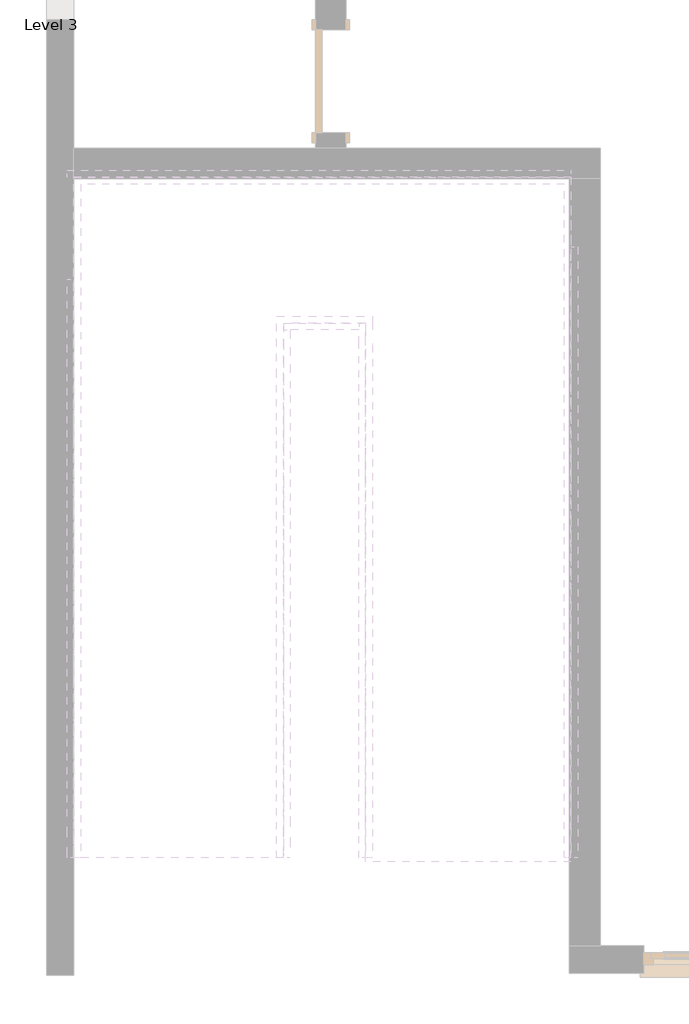
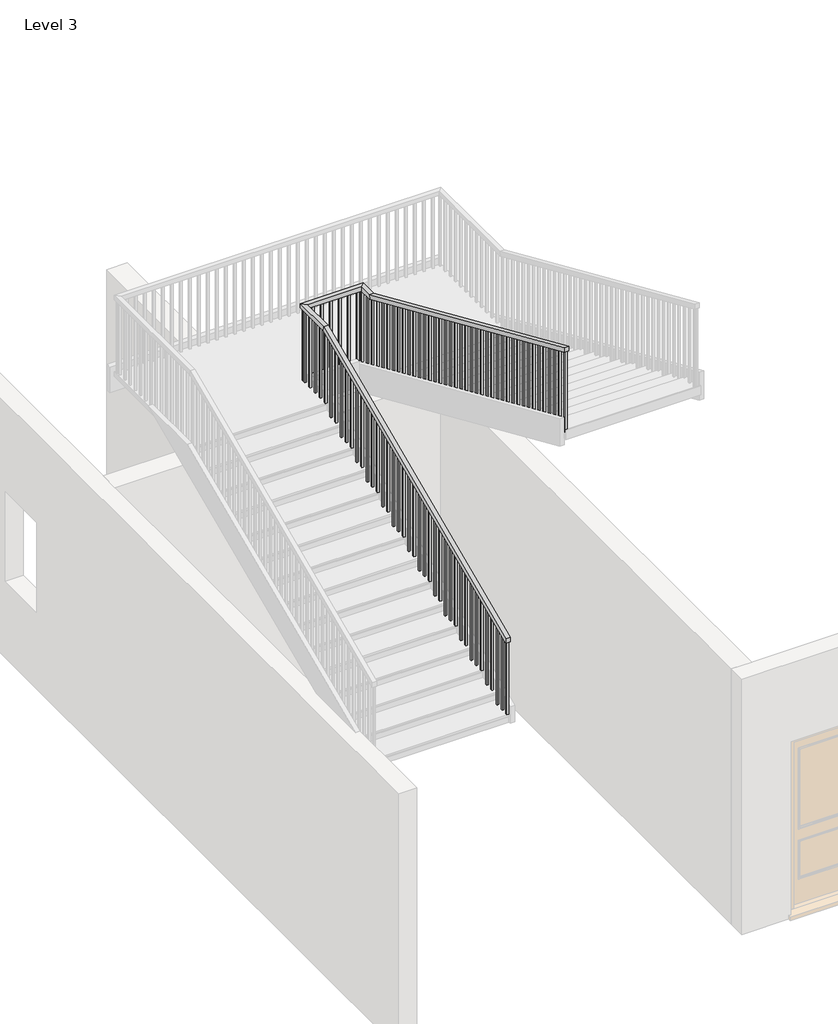
# One storey, part 2 of 6: 1 railing.
"""IFC4 building model written with IfcOpenShell, lengths in millimetres."""

from ifc_helpers import new_model, si_unit, frame, origin, place, context, project, spatial, polyline, outline, extrude, faceted_brep, element, save

model = new_model("IFC4")

# Units and contexts
model_context = context("Model", 3, world=origin())
ifc_project = project(units=[si_unit("LENGTHUNIT", "METRE", prefix="MILLI")], contexts=[model_context])

# Site, building, storey
site = spatial("IfcSite", under=ifc_project)
building = spatial("IfcBuilding", under=site)
storey = spatial("IfcBuildingStorey", under=building, Name="Level 3", Elevation=6096.0)

# Railing
placement = place(None, origin())
element("IfcRailing", 1, ObjectType="Handrail - Rectangular", at=placement, inside=storey, context=model_context, shape_type="SolidModel", body=[
    faceted_brep([(-6050.7290366, -6973.0610642, 9865.36), (-6050.7290366, -6973.0610642, 9809.8599828), (-5999.9290366, -6973.0610642, 9809.8599828), (-5999.9290366, -6973.0610642, 9865.36), (-6050.7290366, -3417.0610642, 11430.0), (-6050.7290366, -3406.3792071, 11379.2), (-5999.9290366, -3406.3792071, 11379.2), (-5999.9290366, -3417.0610642, 11430.0), (-6050.7290366, -2959.8610642, 11430.0), (-6050.7290366, -2959.8610642, 11379.2), (-5999.9290366, -3010.6610642, 11379.2), (-5999.9290366, -3010.6610642, 11430.0), (-5339.5290366, -2959.8610642, 11430.0), (-5339.5290366, -2959.8610642, 11379.2), (-5390.3290366, -3010.6610642, 11379.2), (-5390.3290366, -3010.6610642, 11430.0), (-5339.5290366, -3163.0610642, 11430.0), (-5339.5290366, -3173.7429214, 11379.2), (-5390.3290366, -3173.7429214, 11379.2), (-5390.3290366, -3163.0610642, 11430.0), (-5339.5290366, -6973.0610642, 13106.4), (-5390.3290366, -6973.0610642, 13106.4), (-5390.3290366, -6973.0610642, 13050.8999828), (-5339.5290366, -6973.0610642, 13050.8999828)], [[[0, 1, 2, 3]], [[1, 0, 4, 5]], [[2, 1, 5, 6]], [[3, 2, 6, 7]], [[0, 3, 7, 4]], [[5, 4, 8, 9]], [[6, 5, 9, 10]], [[7, 6, 10, 11]], [[4, 7, 11, 8]], [[9, 8, 12, 13]], [[10, 9, 13, 14]], [[11, 10, 14, 15]], [[8, 11, 15, 12]], [[13, 12, 16, 17]], [[14, 13, 17, 18]], [[15, 14, 18, 19]], [[12, 15, 19, 16]], [[20, 21, 22, 23]], [[17, 16, 20, 23]], [[18, 17, 23, 22]], [[19, 18, 22, 21]], [[16, 19, 21, 20]]]),
    extrude(outline(polyline([(-6957.1860642, 13043.9149828), (-6938.1360642, 13035.5329828), (-6938.1360642, 12080.24), (-6957.1860642, 12080.24), (-6957.1860642, 13043.9149828)])), frame((-5374.4540366, 0.0, 0.0), z_axis=(1.0, 0.0, 0.0), x_axis=(0.0, 1.0, 0.0)), (0.0, 0.0, 1.0), 19.05),
    extrude(outline(polyline([(-6855.5860642, 12999.2109828), (-6836.5360642, 12990.8289828), (-6836.5360642, 12080.24), (-6855.5860642, 12080.24), (-6855.5860642, 12999.2109828)])), frame((-5374.4540366, 0.0, 0.0), z_axis=(1.0, 0.0, 0.0), x_axis=(0.0, 1.0, 0.0)), (0.0, 0.0, 1.0), 19.05),
    extrude(outline(polyline([(-6753.9860642, 12954.5069828), (-6734.9360642, 12946.1249828), (-6734.9360642, 12080.24), (-6753.9860642, 12080.24), (-6753.9860642, 12954.5069828)])), frame((-5374.4540366, 0.0, 0.0), z_axis=(1.0, 0.0, 0.0), x_axis=(0.0, 1.0, 0.0)), (0.0, 0.0, 1.0), 19.05),
    extrude(outline(polyline([(-6652.3860642, 12909.8029828), (-6633.3360642, 12901.4209828), (-6633.3360642, 11968.48), (-6652.3860642, 11968.48), (-6652.3860642, 12909.8029828)])), frame((-5374.4540366, 0.0, 0.0), z_axis=(1.0, 0.0, 0.0), x_axis=(0.0, 1.0, 0.0)), (0.0, 0.0, 1.0), 19.05),
    extrude(outline(polyline([(-6550.7860642, 12865.0989828), (-6531.7360642, 12856.7169828), (-6531.7360642, 11968.48), (-6550.7860642, 11968.48), (-6550.7860642, 12865.0989828)])), frame((-5374.4540366, 0.0, 0.0), z_axis=(1.0, 0.0, 0.0), x_axis=(0.0, 1.0, 0.0)), (0.0, 0.0, 1.0), 19.05),
    extrude(outline(polyline([(-6449.1860642, 12820.3949828), (-6430.1360642, 12812.0129828), (-6430.1360642, 11856.72), (-6449.1860642, 11856.72), (-6449.1860642, 12820.3949828)])), frame((-5374.4540366, 0.0, 0.0), z_axis=(1.0, 0.0, 0.0), x_axis=(0.0, 1.0, 0.0)), (0.0, 0.0, 1.0), 19.05),
    extrude(outline(polyline([(-6347.5860642, 12775.6909828), (-6328.5360642, 12767.3089828), (-6328.5360642, 11856.72), (-6347.5860642, 11856.72), (-6347.5860642, 12775.6909828)])), frame((-5374.4540366, 0.0, 0.0), z_axis=(1.0, 0.0, 0.0), x_axis=(0.0, 1.0, 0.0)), (0.0, 0.0, 1.0), 19.05),
    extrude(outline(polyline([(-6245.9860642, 12730.9869828), (-6226.9360642, 12722.6049828), (-6226.9360642, 11856.72), (-6245.9860642, 11856.72), (-6245.9860642, 12730.9869828)])), frame((-5374.4540366, 0.0, 0.0), z_axis=(1.0, 0.0, 0.0), x_axis=(0.0, 1.0, 0.0)), (0.0, 0.0, 1.0), 19.05),
    extrude(outline(polyline([(-6144.3860642, 12686.2829828), (-6125.3360642, 12677.9009828), (-6125.3360642, 11744.96), (-6144.3860642, 11744.96), (-6144.3860642, 12686.2829828)])), frame((-5374.4540366, 0.0, 0.0), z_axis=(1.0, 0.0, 0.0), x_axis=(0.0, 1.0, 0.0)), (0.0, 0.0, 1.0), 19.05),
    extrude(outline(polyline([(-6042.7860642, 12641.5789828), (-6023.7360642, 12633.1969828), (-6023.7360642, 11744.96), (-6042.7860642, 11744.96), (-6042.7860642, 12641.5789828)])), frame((-5374.4540366, 0.0, 0.0), z_axis=(1.0, 0.0, 0.0), x_axis=(0.0, 1.0, 0.0)), (0.0, 0.0, 1.0), 19.05),
    extrude(outline(polyline([(-5941.1860642, 12596.8749828), (-5922.1360642, 12588.4929828), (-5922.1360642, 11633.2), (-5941.1860642, 11633.2), (-5941.1860642, 12596.8749828)])), frame((-5374.4540366, 0.0, 0.0), z_axis=(1.0, 0.0, 0.0), x_axis=(0.0, 1.0, 0.0)), (0.0, 0.0, 1.0), 19.05),
    extrude(outline(polyline([(-5839.5860642, 12552.1709828), (-5820.5360642, 12543.7889828), (-5820.5360642, 11633.2), (-5839.5860642, 11633.2), (-5839.5860642, 12552.1709828)])), frame((-5374.4540366, 0.0, 0.0), z_axis=(1.0, 0.0, 0.0), x_axis=(0.0, 1.0, 0.0)), (0.0, 0.0, 1.0), 19.05),
    extrude(outline(polyline([(-5737.9860642, 12507.4669828), (-5718.9360642, 12499.0849828), (-5718.9360642, 11633.2), (-5737.9860642, 11633.2), (-5737.9860642, 12507.4669828)])), frame((-5374.4540366, 0.0, 0.0), z_axis=(1.0, 0.0, 0.0), x_axis=(0.0, 1.0, 0.0)), (0.0, 0.0, 1.0), 19.05),
    extrude(outline(polyline([(-5636.3860642, 12462.7629828), (-5617.3360642, 12454.3809828), (-5617.3360642, 11521.44), (-5636.3860642, 11521.44), (-5636.3860642, 12462.7629828)])), frame((-5374.4540366, 0.0, 0.0), z_axis=(1.0, 0.0, 0.0), x_axis=(0.0, 1.0, 0.0)), (0.0, 0.0, 1.0), 19.05),
    extrude(outline(polyline([(-5534.7860642, 12418.0589828), (-5515.7360642, 12409.6769828), (-5515.7360642, 11521.44), (-5534.7860642, 11521.44), (-5534.7860642, 12418.0589828)])), frame((-5374.4540366, 0.0, 0.0), z_axis=(1.0, 0.0, 0.0), x_axis=(0.0, 1.0, 0.0)), (0.0, 0.0, 1.0), 19.05),
    extrude(outline(polyline([(-5433.1860642, 12373.3549828), (-5414.1360642, 12364.9729828), (-5414.1360642, 11409.68), (-5433.1860642, 11409.68), (-5433.1860642, 12373.3549828)])), frame((-5374.4540366, 0.0, 0.0), z_axis=(1.0, 0.0, 0.0), x_axis=(0.0, 1.0, 0.0)), (0.0, 0.0, 1.0), 19.05),
    extrude(outline(polyline([(-5331.5860642, 12328.6509828), (-5312.5360642, 12320.2689828), (-5312.5360642, 11409.68), (-5331.5860642, 11409.68), (-5331.5860642, 12328.6509828)])), frame((-5374.4540366, 0.0, 0.0), z_axis=(1.0, 0.0, 0.0), x_axis=(0.0, 1.0, 0.0)), (0.0, 0.0, 1.0), 19.05),
    extrude(outline(polyline([(-5229.9860642, 12283.9469828), (-5210.9360642, 12275.5649828), (-5210.9360642, 11409.68), (-5229.9860642, 11409.68), (-5229.9860642, 12283.9469828)])), frame((-5374.4540366, 0.0, 0.0), z_axis=(1.0, 0.0, 0.0), x_axis=(0.0, 1.0, 0.0)), (0.0, 0.0, 1.0), 19.05),
    extrude(outline(polyline([(-5128.3860642, 12239.2429828), (-5109.3360642, 12230.8609828), (-5109.3360642, 11297.92), (-5128.3860642, 11297.92), (-5128.3860642, 12239.2429828)])), frame((-5374.4540366, 0.0, 0.0), z_axis=(1.0, 0.0, 0.0), x_axis=(0.0, 1.0, 0.0)), (0.0, 0.0, 1.0), 19.05),
    extrude(outline(polyline([(-5026.7860642, 12194.5389828), (-5007.7360642, 12186.1569828), (-5007.7360642, 11297.92), (-5026.7860642, 11297.92), (-5026.7860642, 12194.5389828)])), frame((-5374.4540366, 0.0, 0.0), z_axis=(1.0, 0.0, 0.0), x_axis=(0.0, 1.0, 0.0)), (0.0, 0.0, 1.0), 19.05),
    extrude(outline(polyline([(-4925.1860642, 12149.8349828), (-4906.1360642, 12141.4529828), (-4906.1360642, 11186.16), (-4925.1860642, 11186.16), (-4925.1860642, 12149.8349828)])), frame((-5374.4540366, 0.0, 0.0), z_axis=(1.0, 0.0, 0.0), x_axis=(0.0, 1.0, 0.0)), (0.0, 0.0, 1.0), 19.05),
    extrude(outline(polyline([(-4823.5860642, 12105.1309828), (-4804.5360642, 12096.7489828), (-4804.5360642, 11186.16), (-4823.5860642, 11186.16), (-4823.5860642, 12105.1309828)])), frame((-5374.4540366, 0.0, 0.0), z_axis=(1.0, 0.0, 0.0), x_axis=(0.0, 1.0, 0.0)), (0.0, 0.0, 1.0), 19.05),
    extrude(outline(polyline([(-4721.9860642, 12060.4269828), (-4702.9360642, 12052.0449828), (-4702.9360642, 11186.16), (-4721.9860642, 11186.16), (-4721.9860642, 12060.4269828)])), frame((-5374.4540366, 0.0, 0.0), z_axis=(1.0, 0.0, 0.0), x_axis=(0.0, 1.0, 0.0)), (0.0, 0.0, 1.0), 19.05),
    extrude(outline(polyline([(-4620.3860642, 12015.7229828), (-4601.3360642, 12007.3409828), (-4601.3360642, 11074.4), (-4620.3860642, 11074.4), (-4620.3860642, 12015.7229828)])), frame((-5374.4540366, 0.0, 0.0), z_axis=(1.0, 0.0, 0.0), x_axis=(0.0, 1.0, 0.0)), (0.0, 0.0, 1.0), 19.05),
    extrude(outline(polyline([(-4518.7860642, 11971.0189828), (-4499.7360642, 11962.6369828), (-4499.7360642, 11074.4), (-4518.7860642, 11074.4), (-4518.7860642, 11971.0189828)])), frame((-5374.4540366, 0.0, 0.0), z_axis=(1.0, 0.0, 0.0), x_axis=(0.0, 1.0, 0.0)), (0.0, 0.0, 1.0), 19.05),
    extrude(outline(polyline([(-4417.1860642, 11926.3149828), (-4398.1360642, 11917.9329828), (-4398.1360642, 10962.64), (-4417.1860642, 10962.64), (-4417.1860642, 11926.3149828)])), frame((-5374.4540366, 0.0, 0.0), z_axis=(1.0, 0.0, 0.0), x_axis=(0.0, 1.0, 0.0)), (0.0, 0.0, 1.0), 19.05),
    extrude(outline(polyline([(-4315.5860642, 11881.6109828), (-4296.5360642, 11873.2289828), (-4296.5360642, 10962.64), (-4315.5860642, 10962.64), (-4315.5860642, 11881.6109828)])), frame((-5374.4540366, 0.0, 0.0), z_axis=(1.0, 0.0, 0.0), x_axis=(0.0, 1.0, 0.0)), (0.0, 0.0, 1.0), 19.05),
    extrude(outline(polyline([(-4213.9860642, 11836.9069828), (-4194.9360642, 11828.5249828), (-4194.9360642, 10962.64), (-4213.9860642, 10962.64), (-4213.9860642, 11836.9069828)])), frame((-5374.4540366, 0.0, 0.0), z_axis=(1.0, 0.0, 0.0), x_axis=(0.0, 1.0, 0.0)), (0.0, 0.0, 1.0), 19.05),
    extrude(outline(polyline([(-4112.3860642, 11792.2029828), (-4093.3360642, 11783.8209828), (-4093.3360642, 10850.88), (-4112.3860642, 10850.88), (-4112.3860642, 11792.2029828)])), frame((-5374.4540366, 0.0, 0.0), z_axis=(1.0, 0.0, 0.0), x_axis=(0.0, 1.0, 0.0)), (0.0, 0.0, 1.0), 19.05),
    extrude(outline(polyline([(-4010.7860642, 11747.4989828), (-3991.7360642, 11739.1169828), (-3991.7360642, 10850.88), (-4010.7860642, 10850.88), (-4010.7860642, 11747.4989828)])), frame((-5374.4540366, 0.0, 0.0), z_axis=(1.0, 0.0, 0.0), x_axis=(0.0, 1.0, 0.0)), (0.0, 0.0, 1.0), 19.05),
    extrude(outline(polyline([(-3909.1860642, 11702.7949828), (-3890.1360642, 11694.4129828), (-3890.1360642, 10739.12), (-3909.1860642, 10739.12), (-3909.1860642, 11702.7949828)])), frame((-5374.4540366, 0.0, 0.0), z_axis=(1.0, 0.0, 0.0), x_axis=(0.0, 1.0, 0.0)), (0.0, 0.0, 1.0), 19.05),
    extrude(outline(polyline([(-3807.5860642, 11658.0909828), (-3788.5360642, 11649.7089828), (-3788.5360642, 10739.12), (-3807.5860642, 10739.12), (-3807.5860642, 11658.0909828)])), frame((-5374.4540366, 0.0, 0.0), z_axis=(1.0, 0.0, 0.0), x_axis=(0.0, 1.0, 0.0)), (0.0, 0.0, 1.0), 19.05),
    extrude(outline(polyline([(-3705.9860642, 11613.3869828), (-3686.9360642, 11605.0049828), (-3686.9360642, 10739.12), (-3705.9860642, 10739.12), (-3705.9860642, 11613.3869828)])), frame((-5374.4540366, 0.0, 0.0), z_axis=(1.0, 0.0, 0.0), x_axis=(0.0, 1.0, 0.0)), (0.0, 0.0, 1.0), 19.05),
    extrude(outline(polyline([(-3604.3860642, 11568.6829828), (-3585.3360642, 11560.3009828), (-3585.3360642, 10627.36), (-3604.3860642, 10627.36), (-3604.3860642, 11568.6829828)])), frame((-5374.4540366, 0.0, 0.0), z_axis=(1.0, 0.0, 0.0), x_axis=(0.0, 1.0, 0.0)), (0.0, 0.0, 1.0), 19.05),
    extrude(outline(polyline([(-3502.7860642, 11523.9789828), (-3483.7360642, 11515.5969828), (-3483.7360642, 10627.36), (-3502.7860642, 10627.36), (-3502.7860642, 11523.9789828)])), frame((-5374.4540366, 0.0, 0.0), z_axis=(1.0, 0.0, 0.0), x_axis=(0.0, 1.0, 0.0)), (0.0, 0.0, 1.0), 19.05),
    extrude(outline(polyline([(-3401.1860642, 11479.2749828), (-3382.1360642, 11470.8929828), (-3382.1360642, 10515.6), (-3401.1860642, 10515.6), (-3401.1860642, 11479.2749828)])), frame((-5374.4540366, 0.0, 0.0), z_axis=(1.0, 0.0, 0.0), x_axis=(0.0, 1.0, 0.0)), (0.0, 0.0, 1.0), 19.05),
    extrude(outline(polyline([(-3299.5860642, 11434.5709828), (-3280.5360642, 11426.1889828), (-3280.5360642, 10515.6), (-3299.5860642, 10515.6), (-3299.5860642, 11434.5709828)])), frame((-5374.4540366, 0.0, 0.0), z_axis=(1.0, 0.0, 0.0), x_axis=(0.0, 1.0, 0.0)), (0.0, 0.0, 1.0), 19.05),
    extrude(outline(polyline([(-3197.9860642, 11389.8669828), (-3178.9360642, 11381.4849828), (-3178.9360642, 10515.6), (-3197.9860642, 10515.6), (-3197.9860642, 11389.8669828)])), frame((-5374.4540366, 0.0, 0.0), z_axis=(1.0, 0.0, 0.0), x_axis=(0.0, 1.0, 0.0)), (0.0, 0.0, 1.0), 19.05),
    extrude(outline(polyline([(-5374.4540366, -3077.3360642), (-5355.4040366, -3077.3360642), (-5355.4040366, -3096.3860642), (-5374.4540366, -3096.3860642), (-5374.4540366, -3077.3360642)])), frame((0.0, 0.0, 10515.6), z_axis=(0.0, 0.0, 1.0), x_axis=(1.0, 0.0, 0.0)), (0.0, 0.0, 1.0), 863.6),
    extrude(outline(polyline([(-5425.2540366, -2994.7860642), (-5425.2540366, -2975.7360642), (-5406.2040366, -2975.7360642), (-5406.2040366, -2994.7860642), (-5425.2540366, -2994.7860642)])), frame((0.0, 0.0, 10515.6), z_axis=(0.0, 0.0, 1.0), x_axis=(1.0, 0.0, 0.0)), (0.0, 0.0, 1.0), 863.6),
    extrude(outline(polyline([(-5526.8540366, -2994.7860642), (-5526.8540366, -2975.7360642), (-5507.8040366, -2975.7360642), (-5507.8040366, -2994.7860642), (-5526.8540366, -2994.7860642)])), frame((0.0, 0.0, 10515.6), z_axis=(0.0, 0.0, 1.0), x_axis=(1.0, 0.0, 0.0)), (0.0, 0.0, 1.0), 863.6),
    extrude(outline(polyline([(-5628.4540366, -2994.7860642), (-5628.4540366, -2975.7360642), (-5609.4040366, -2975.7360642), (-5609.4040366, -2994.7860642), (-5628.4540366, -2994.7860642)])), frame((0.0, 0.0, 10515.6), z_axis=(0.0, 0.0, 1.0), x_axis=(1.0, 0.0, 0.0)), (0.0, 0.0, 1.0), 863.6),
    extrude(outline(polyline([(-5730.0540366, -2994.7860642), (-5730.0540366, -2975.7360642), (-5711.0040366, -2975.7360642), (-5711.0040366, -2994.7860642), (-5730.0540366, -2994.7860642)])), frame((0.0, 0.0, 10515.6), z_axis=(0.0, 0.0, 1.0), x_axis=(1.0, 0.0, 0.0)), (0.0, 0.0, 1.0), 863.6),
    extrude(outline(polyline([(-5831.6540366, -2994.7860642), (-5831.6540366, -2975.7360642), (-5812.6040366, -2975.7360642), (-5812.6040366, -2994.7860642), (-5831.6540366, -2994.7860642)])), frame((0.0, 0.0, 10515.6), z_axis=(0.0, 0.0, 1.0), x_axis=(1.0, 0.0, 0.0)), (0.0, 0.0, 1.0), 863.6),
    extrude(outline(polyline([(-5933.2540366, -2994.7860642), (-5933.2540366, -2975.7360642), (-5914.2040366, -2975.7360642), (-5914.2040366, -2994.7860642), (-5933.2540366, -2994.7860642)])), frame((0.0, 0.0, 10515.6), z_axis=(0.0, 0.0, 1.0), x_axis=(1.0, 0.0, 0.0)), (0.0, 0.0, 1.0), 863.6),
    extrude(outline(polyline([(-6015.8040366, -3020.1860642), (-6034.8540366, -3020.1860642), (-6034.8540366, -3001.1360642), (-6015.8040366, -3001.1360642), (-6015.8040366, -3020.1860642)])), frame((0.0, 0.0, 10515.6), z_axis=(0.0, 0.0, 1.0), x_axis=(1.0, 0.0, 0.0)), (0.0, 0.0, 1.0), 863.6),
    extrude(outline(polyline([(-6015.8040366, -3121.7860642), (-6034.8540366, -3121.7860642), (-6034.8540366, -3102.7360642), (-6015.8040366, -3102.7360642), (-6015.8040366, -3121.7860642)])), frame((0.0, 0.0, 10515.6), z_axis=(0.0, 0.0, 1.0), x_axis=(1.0, 0.0, 0.0)), (0.0, 0.0, 1.0), 863.6),
    extrude(outline(polyline([(-6015.8040366, -3223.3860642), (-6034.8540366, -3223.3860642), (-6034.8540366, -3204.3360642), (-6015.8040366, -3204.3360642), (-6015.8040366, -3223.3860642)])), frame((0.0, 0.0, 10515.6), z_axis=(0.0, 0.0, 1.0), x_axis=(1.0, 0.0, 0.0)), (0.0, 0.0, 1.0), 863.6),
    extrude(outline(polyline([(-6015.8040366, -3324.9860642), (-6034.8540366, -3324.9860642), (-6034.8540366, -3305.9360642), (-6015.8040366, -3305.9360642), (-6015.8040366, -3324.9860642)])), frame((0.0, 0.0, 10515.6), z_axis=(0.0, 0.0, 1.0), x_axis=(1.0, 0.0, 0.0)), (0.0, 0.0, 1.0), 863.6),
    extrude(outline(polyline([(-3426.5860642, 11370.3089828), (-3407.5360642, 11378.6909828), (-3407.5360642, 10515.6), (-3426.5860642, 10515.6), (-3426.5860642, 11370.3089828)])), frame((-6034.8540366, 0.0, 0.0), z_axis=(1.0, 0.0, 0.0), x_axis=(0.0, 1.0, 0.0)), (0.0, 0.0, 1.0), 19.05),
    extrude(outline(polyline([(-3528.1860642, 11325.6049828), (-3509.1360642, 11333.9869828), (-3509.1360642, 10403.84), (-3528.1860642, 10403.84), (-3528.1860642, 11325.6049828)])), frame((-6034.8540366, 0.0, 0.0), z_axis=(1.0, 0.0, 0.0), x_axis=(0.0, 1.0, 0.0)), (0.0, 0.0, 1.0), 19.05),
    extrude(outline(polyline([(-3629.7860642, 11280.9009828), (-3610.7360642, 11289.2829828), (-3610.7360642, 10403.84), (-3629.7860642, 10403.84), (-3629.7860642, 11280.9009828)])), frame((-6034.8540366, 0.0, 0.0), z_axis=(1.0, 0.0, 0.0), x_axis=(0.0, 1.0, 0.0)), (0.0, 0.0, 1.0), 19.05),
    extrude(outline(polyline([(-3731.3860642, 11236.1969828), (-3712.3360642, 11244.5789828), (-3712.3360642, 10292.08), (-3731.3860642, 10292.08), (-3731.3860642, 11236.1969828)])), frame((-6034.8540366, 0.0, 0.0), z_axis=(1.0, 0.0, 0.0), x_axis=(0.0, 1.0, 0.0)), (0.0, 0.0, 1.0), 19.05),
    extrude(outline(polyline([(-3832.9860642, 11191.4929828), (-3813.9360642, 11199.8749828), (-3813.9360642, 10292.08), (-3832.9860642, 10292.08), (-3832.9860642, 11191.4929828)])), frame((-6034.8540366, 0.0, 0.0), z_axis=(1.0, 0.0, 0.0), x_axis=(0.0, 1.0, 0.0)), (0.0, 0.0, 1.0), 19.05),
    extrude(outline(polyline([(-3934.5860642, 11146.7889828), (-3915.5360642, 11155.1709828), (-3915.5360642, 10292.08), (-3934.5860642, 10292.08), (-3934.5860642, 11146.7889828)])), frame((-6034.8540366, 0.0, 0.0), z_axis=(1.0, 0.0, 0.0), x_axis=(0.0, 1.0, 0.0)), (0.0, 0.0, 1.0), 19.05),
    extrude(outline(polyline([(-4036.1860642, 11102.0849828), (-4017.1360642, 11110.4669828), (-4017.1360642, 10180.32), (-4036.1860642, 10180.32), (-4036.1860642, 11102.0849828)])), frame((-6034.8540366, 0.0, 0.0), z_axis=(1.0, 0.0, 0.0), x_axis=(0.0, 1.0, 0.0)), (0.0, 0.0, 1.0), 19.05),
    extrude(outline(polyline([(-4137.7860642, 11057.3809828), (-4118.7360642, 11065.7629828), (-4118.7360642, 10180.32), (-4137.7860642, 10180.32), (-4137.7860642, 11057.3809828)])), frame((-6034.8540366, 0.0, 0.0), z_axis=(1.0, 0.0, 0.0), x_axis=(0.0, 1.0, 0.0)), (0.0, 0.0, 1.0), 19.05),
    extrude(outline(polyline([(-4239.3860642, 11012.6769828), (-4220.3360642, 11021.0589828), (-4220.3360642, 10068.56), (-4239.3860642, 10068.56), (-4239.3860642, 11012.6769828)])), frame((-6034.8540366, 0.0, 0.0), z_axis=(1.0, 0.0, 0.0), x_axis=(0.0, 1.0, 0.0)), (0.0, 0.0, 1.0), 19.05),
    extrude(outline(polyline([(-4340.9860642, 10967.9729828), (-4321.9360642, 10976.3549828), (-4321.9360642, 10068.56), (-4340.9860642, 10068.56), (-4340.9860642, 10967.9729828)])), frame((-6034.8540366, 0.0, 0.0), z_axis=(1.0, 0.0, 0.0), x_axis=(0.0, 1.0, 0.0)), (0.0, 0.0, 1.0), 19.05),
    extrude(outline(polyline([(-4442.5860642, 10923.2689828), (-4423.5360642, 10931.6509828), (-4423.5360642, 10068.56), (-4442.5860642, 10068.56), (-4442.5860642, 10923.2689828)])), frame((-6034.8540366, 0.0, 0.0), z_axis=(1.0, 0.0, 0.0), x_axis=(0.0, 1.0, 0.0)), (0.0, 0.0, 1.0), 19.05),
    extrude(outline(polyline([(-4544.1860642, 10878.5649828), (-4525.1360642, 10886.9469828), (-4525.1360642, 9956.8), (-4544.1860642, 9956.8), (-4544.1860642, 10878.5649828)])), frame((-6034.8540366, 0.0, 0.0), z_axis=(1.0, 0.0, 0.0), x_axis=(0.0, 1.0, 0.0)), (0.0, 0.0, 1.0), 19.05),
    extrude(outline(polyline([(-4645.7860642, 10833.8609828), (-4626.7360642, 10842.2429828), (-4626.7360642, 9956.8), (-4645.7860642, 9956.8), (-4645.7860642, 10833.8609828)])), frame((-6034.8540366, 0.0, 0.0), z_axis=(1.0, 0.0, 0.0), x_axis=(0.0, 1.0, 0.0)), (0.0, 0.0, 1.0), 19.05),
    extrude(outline(polyline([(-4747.3860642, 10789.1569828), (-4728.3360642, 10797.5389828), (-4728.3360642, 9845.04), (-4747.3860642, 9845.04), (-4747.3860642, 10789.1569828)])), frame((-6034.8540366, 0.0, 0.0), z_axis=(1.0, 0.0, 0.0), x_axis=(0.0, 1.0, 0.0)), (0.0, 0.0, 1.0), 19.05),
    extrude(outline(polyline([(-4848.9860642, 10744.4529828), (-4829.9360642, 10752.8349828), (-4829.9360642, 9845.04), (-4848.9860642, 9845.04), (-4848.9860642, 10744.4529828)])), frame((-6034.8540366, 0.0, 0.0), z_axis=(1.0, 0.0, 0.0), x_axis=(0.0, 1.0, 0.0)), (0.0, 0.0, 1.0), 19.05),
    extrude(outline(polyline([(-4950.5860642, 10699.7489828), (-4931.5360642, 10708.1309828), (-4931.5360642, 9845.04), (-4950.5860642, 9845.04), (-4950.5860642, 10699.7489828)])), frame((-6034.8540366, 0.0, 0.0), z_axis=(1.0, 0.0, 0.0), x_axis=(0.0, 1.0, 0.0)), (0.0, 0.0, 1.0), 19.05),
    extrude(outline(polyline([(-5052.1860642, 10655.0449828), (-5033.1360642, 10663.4269828), (-5033.1360642, 9733.28), (-5052.1860642, 9733.28), (-5052.1860642, 10655.0449828)])), frame((-6034.8540366, 0.0, 0.0), z_axis=(1.0, 0.0, 0.0), x_axis=(0.0, 1.0, 0.0)), (0.0, 0.0, 1.0), 19.05),
    extrude(outline(polyline([(-5153.7860642, 10610.3409828), (-5134.7360642, 10618.7229828), (-5134.7360642, 9733.28), (-5153.7860642, 9733.28), (-5153.7860642, 10610.3409828)])), frame((-6034.8540366, 0.0, 0.0), z_axis=(1.0, 0.0, 0.0), x_axis=(0.0, 1.0, 0.0)), (0.0, 0.0, 1.0), 19.05),
    extrude(outline(polyline([(-5255.3860642, 10565.6369828), (-5236.3360642, 10574.0189828), (-5236.3360642, 9621.52), (-5255.3860642, 9621.52), (-5255.3860642, 10565.6369828)])), frame((-6034.8540366, 0.0, 0.0), z_axis=(1.0, 0.0, 0.0), x_axis=(0.0, 1.0, 0.0)), (0.0, 0.0, 1.0), 19.05),
    extrude(outline(polyline([(-5356.9860642, 10520.9329828), (-5337.9360642, 10529.3149828), (-5337.9360642, 9621.52), (-5356.9860642, 9621.52), (-5356.9860642, 10520.9329828)])), frame((-6034.8540366, 0.0, 0.0), z_axis=(1.0, 0.0, 0.0), x_axis=(0.0, 1.0, 0.0)), (0.0, 0.0, 1.0), 19.05),
    extrude(outline(polyline([(-5458.5860642, 10476.2289828), (-5439.5360642, 10484.6109828), (-5439.5360642, 9621.52), (-5458.5860642, 9621.52), (-5458.5860642, 10476.2289828)])), frame((-6034.8540366, 0.0, 0.0), z_axis=(1.0, 0.0, 0.0), x_axis=(0.0, 1.0, 0.0)), (0.0, 0.0, 1.0), 19.05),
    extrude(outline(polyline([(-5560.1860642, 10431.5249828), (-5541.1360642, 10439.9069828), (-5541.1360642, 9509.76), (-5560.1860642, 9509.76), (-5560.1860642, 10431.5249828)])), frame((-6034.8540366, 0.0, 0.0), z_axis=(1.0, 0.0, 0.0), x_axis=(0.0, 1.0, 0.0)), (0.0, 0.0, 1.0), 19.05),
    extrude(outline(polyline([(-5661.7860642, 10386.8209828), (-5642.7360642, 10395.2029828), (-5642.7360642, 9509.76), (-5661.7860642, 9509.76), (-5661.7860642, 10386.8209828)])), frame((-6034.8540366, 0.0, 0.0), z_axis=(1.0, 0.0, 0.0), x_axis=(0.0, 1.0, 0.0)), (0.0, 0.0, 1.0), 19.05),
    extrude(outline(polyline([(-5763.3860642, 10342.1169828), (-5744.3360642, 10350.4989828), (-5744.3360642, 9398.0), (-5763.3860642, 9398.0), (-5763.3860642, 10342.1169828)])), frame((-6034.8540366, 0.0, 0.0), z_axis=(1.0, 0.0, 0.0), x_axis=(0.0, 1.0, 0.0)), (0.0, 0.0, 1.0), 19.05),
    extrude(outline(polyline([(-5864.9860642, 10297.4129828), (-5845.9360642, 10305.7949828), (-5845.9360642, 9398.0), (-5864.9860642, 9398.0), (-5864.9860642, 10297.4129828)])), frame((-6034.8540366, 0.0, 0.0), z_axis=(1.0, 0.0, 0.0), x_axis=(0.0, 1.0, 0.0)), (0.0, 0.0, 1.0), 19.05),
    extrude(outline(polyline([(-5966.5860642, 10252.7089828), (-5947.5360642, 10261.0909828), (-5947.5360642, 9398.0), (-5966.5860642, 9398.0), (-5966.5860642, 10252.7089828)])), frame((-6034.8540366, 0.0, 0.0), z_axis=(1.0, 0.0, 0.0), x_axis=(0.0, 1.0, 0.0)), (0.0, 0.0, 1.0), 19.05),
    extrude(outline(polyline([(-6068.1860642, 10208.0049828), (-6049.1360642, 10216.3869828), (-6049.1360642, 9286.24), (-6068.1860642, 9286.24), (-6068.1860642, 10208.0049828)])), frame((-6034.8540366, 0.0, 0.0), z_axis=(1.0, 0.0, 0.0), x_axis=(0.0, 1.0, 0.0)), (0.0, 0.0, 1.0), 19.05),
    extrude(outline(polyline([(-6169.7860642, 10163.3009828), (-6150.7360642, 10171.6829828), (-6150.7360642, 9286.24), (-6169.7860642, 9286.24), (-6169.7860642, 10163.3009828)])), frame((-6034.8540366, 0.0, 0.0), z_axis=(1.0, 0.0, 0.0), x_axis=(0.0, 1.0, 0.0)), (0.0, 0.0, 1.0), 19.05),
    extrude(outline(polyline([(-6271.3860642, 10118.5969828), (-6252.3360642, 10126.9789828), (-6252.3360642, 9174.48), (-6271.3860642, 9174.48), (-6271.3860642, 10118.5969828)])), frame((-6034.8540366, 0.0, 0.0), z_axis=(1.0, 0.0, 0.0), x_axis=(0.0, 1.0, 0.0)), (0.0, 0.0, 1.0), 19.05),
    extrude(outline(polyline([(-6372.9860642, 10073.8929828), (-6353.9360642, 10082.2749828), (-6353.9360642, 9174.48), (-6372.9860642, 9174.48), (-6372.9860642, 10073.8929828)])), frame((-6034.8540366, 0.0, 0.0), z_axis=(1.0, 0.0, 0.0), x_axis=(0.0, 1.0, 0.0)), (0.0, 0.0, 1.0), 19.05),
    extrude(outline(polyline([(-6474.5860642, 10029.1889828), (-6455.5360642, 10037.5709828), (-6455.5360642, 9174.48), (-6474.5860642, 9174.48), (-6474.5860642, 10029.1889828)])), frame((-6034.8540366, 0.0, 0.0), z_axis=(1.0, 0.0, 0.0), x_axis=(0.0, 1.0, 0.0)), (0.0, 0.0, 1.0), 19.05),
    extrude(outline(polyline([(-6576.1860642, 9984.4849828), (-6557.1360642, 9992.8669828), (-6557.1360642, 9062.72), (-6576.1860642, 9062.72), (-6576.1860642, 9984.4849828)])), frame((-6034.8540366, 0.0, 0.0), z_axis=(1.0, 0.0, 0.0), x_axis=(0.0, 1.0, 0.0)), (0.0, 0.0, 1.0), 19.05),
    extrude(outline(polyline([(-6677.7860642, 9939.7809828), (-6658.7360642, 9948.1629828), (-6658.7360642, 9062.72), (-6677.7860642, 9062.72), (-6677.7860642, 9939.7809828)])), frame((-6034.8540366, 0.0, 0.0), z_axis=(1.0, 0.0, 0.0), x_axis=(0.0, 1.0, 0.0)), (0.0, 0.0, 1.0), 19.05),
    extrude(outline(polyline([(-6779.3860642, 9895.0769828), (-6760.3360642, 9903.4589828), (-6760.3360642, 8950.96), (-6779.3860642, 8950.96), (-6779.3860642, 9895.0769828)])), frame((-6034.8540366, 0.0, 0.0), z_axis=(1.0, 0.0, 0.0), x_axis=(0.0, 1.0, 0.0)), (0.0, 0.0, 1.0), 19.05),
    extrude(outline(polyline([(-6880.9860642, 9850.3729828), (-6861.9360642, 9858.7549828), (-6861.9360642, 8950.96), (-6880.9860642, 8950.96), (-6880.9860642, 9850.3729828)])), frame((-6034.8540366, 0.0, 0.0), z_axis=(1.0, 0.0, 0.0), x_axis=(0.0, 1.0, 0.0)), (0.0, 0.0, 1.0), 19.05),
    extrude(outline(polyline([(-5374.4540366, -2994.7860642), (-5374.4540366, -2975.7360642), (-5355.4040366, -2975.7360642), (-5355.4040366, -2994.7860642), (-5374.4540366, -2994.7860642)])), frame((0.0, 0.0, 10515.6), z_axis=(0.0, 0.0, 1.0), x_axis=(1.0, 0.0, 0.0)), (0.0, 0.0, 1.0), 863.6),
    extrude(outline(polyline([(-6015.8040366, -2994.7860642), (-6034.8540366, -2994.7860642), (-6034.8540366, -2975.7360642), (-6015.8040366, -2975.7360642), (-6015.8040366, -2994.7860642)])), frame((0.0, 0.0, 10515.6), z_axis=(0.0, 0.0, 1.0), x_axis=(1.0, 0.0, 0.0)), (0.0, 0.0, 1.0), 863.6),
    extrude(outline(polyline([(-6973.0610642, 13050.8999828), (-6954.0110642, 13042.5179828), (-6954.0110642, 12080.24), (-6973.0610642, 12080.24), (-6973.0610642, 13050.8999828)])), frame((-5374.4540366, 0.0, 0.0), z_axis=(1.0, 0.0, 0.0), x_axis=(0.0, 1.0, 0.0)), (0.0, 0.0, 1.0), 19.05),
    extrude(outline(polyline([(-6973.0610642, 9809.8599828), (-6954.0110642, 9818.2419828), (-6954.0110642, 8950.96), (-6973.0610642, 8950.96), (-6973.0610642, 9809.8599828)])), frame((-6034.8540366, 0.0, 0.0), z_axis=(1.0, 0.0, 0.0), x_axis=(0.0, 1.0, 0.0)), (0.0, 0.0, 1.0), 19.05),
])

save(model, "model.ifc")

# Revit data of these elements
# Type "Handrail - Rectangular"
#   Assembly Code = "C2010400"
#   built-in parameter 1008612 = 0.0416667 (stored number, unit not read)
#   built-in parameter 1008611 = 0.0416667 (stored number, unit not read)
#   built-in parameter 1008609 = 0.333333 (stored number, unit not read)
#   built-in parameter 1008604 = 0.166667 (stored number, unit not read)
#   built-in parameter 1008603 = 0.166667 (stored number, unit not read)
#   Railing Height = 3' - 0"
#   built-in parameter 1008630 = 2
#   built-in parameter 1008610 = 2
#   built-in parameter 1008618 = Baluster - Square : 3/4"
# Element 1 (IfcRailing, "Handrail - Rectangular")
#   Phase Created = New Construction
